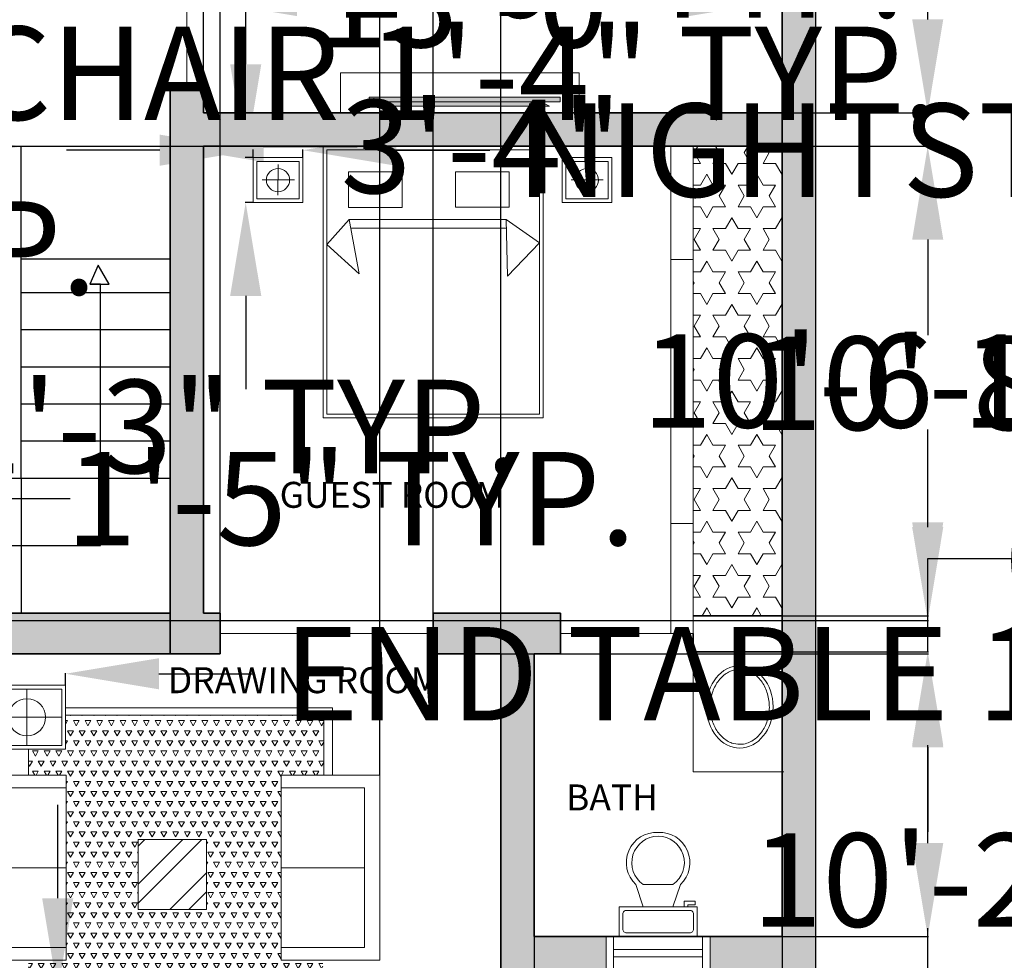
# Model space of a CAD drawing. Units: inches. Extents: x 29 to 6336, y 3 to 2592.
# Tile 6 of 8: x 5672 to 5938, y 2100 to 2354. Entities that reach past the tile are written whole.
import ezdxf

# ---------------------------------------------------------------- set-up
doc = ezdxf.new("R2010")
doc.units = ezdxf.units.IN
doc.header["$MEASUREMENT"] = 0
for name, color, linetype, lineweight in [('A-ANNO-DIMS', 2, 'Continuous', 18), ('A-AREA-IDEN', 7, 'Continuous', 18), ('A-DOOR', 4, 'Continuous', 18), ('A-FLOR-CASE', 8, 'Continuous', 18), ('A-FLOR-FIXT', 8, 'Continuous', 18), ('A-FLOR-FIXT-PATT', 9, 'Continuous', 13), ('A-FLOR-PATT', 9, 'Continuous', 13), ('A-FLOR-STRS', 7, 'Continuous', 25), ('A-FURN', 8, 'Continuous', 18), ('A-FURN-PATT', 18, 'Continuous', 13), ('A-GLAZ', 116, 'Continuous', 18), ('A-WALL', 7, 'Continuous', 35), ('A-WALL-PATT', 242, 'Continuous', 13), ('C-PROP', 7, 'Continuous', 25)]:
    doc.layers.add(name, color=color, linetype=linetype, lineweight=lineweight)
doc.styles.get("Standard").update_dxf_attribs({"font": 'arial.ttf'})
doc.dimstyles.get("Standard").update_dxf_attribs({"dimtxt": 25.18, "dimasz": 25.18, "dimexe": 0.18, "dimexo": 0.0625, "dimgap": 0.09, "dimtad": 0, "dimtih": 1, "dimtoh": 1, "dimdec": 0, "dimzin": 0, "dimdsep": 46, "dimlunit": 3, "dimtxsty": 'Standard', "dimcen": 0.09, "dimadec": 0, "dimazin": 0, "dimtfac": 1, "dimtdec": 0, "dimtofl": 0, "dimtmove": 0, "dimatfit": 3, "dimfxl": 1, "dimtolj": 1, "dimtzin": 0, "dimarcsym": 0})

# ---------------------------------------------------------------- blocks, each defined once
blk = doc.blocks.new('*U4')
for p, q in [((9.5, -6), (9.5, -2)), ((-10, -8.5), (-8, -8.5)), ((-10, -9.5), (-10, -8.5)), ((-7, -9.5), (-10, -9.5)), ((-8, -8.5), (-8, -8)), ((-7, -8), (-7, -9.5)), ((-4, -8), (-6, -14)), ((4, -8), (6, -14)), ((4, -14), (-4, -14))]:
    blk.add_line(p, q)
blk.add_lwpolyline([(10.5, -8), (10.5, 0), (-10.5, 0), (-10.5, -8)], close=True)
for points in [[(-9.5, -2), (-9.5, -6)], [(8.5, -1), (-8.5, -1)], [(-8.5, -7), (8.5, -7)]]:
    blk.add_lwpolyline(points)
for centre, radius, start, end in [((-8.625, -1.875), 0.8839, 81.8699, 188.1301), ((8.625, -1.875), 0.8839, 351.8699, 98.1301), ((-8.625, -6.125), 0.8839, 171.869898, 278.1301), ((8.625, -6.125), 0.8839, 261.8699, 8.1301), ((-0.4772, -19.9188), 8.0953, 133.01722, 273.38), ((0.0374, -19.8731), 7.127, 124.50543, 269.7), ((-0.0373, -19.8731), 7.127, 270.3, 55.4946), ((0.4773, -19.9188), 8.0953, 266.62, 46.9828)]:
    blk.add_arc(centre, radius, start, end)
blk = doc.blocks.new('WIN-24')
for p, q in [((0, 9), (0, 0)), ((2, 9), (2, 0)), ((26, 9), (26, 0)), ((28, 9), (28, 0)), ((2, 5.5), (26, 5.5)), ((2, 3.5), (26, 3.5))]:
    blk.add_line(p, q)
blk = doc.blocks.new('SOFA-TWO-SEAT')
blk.add_line((4.12, 24.97), (26.62, 24.97))
for points in [[(4.17, 49.94), (0, 49.94), (0, 0), (4.17, 0)], [(4.17, 49.94), (26.62, 49.94), (26.62, 46.51), (4.17, 46.51)], [(4.17, 3.43), (4.17, 46.51)], [(4.12, 3.43), (26.57, 3.43), (26.57, 0), (4.12, 0)]]:
    blk.add_lwpolyline(points)
blk.add_lwpolyline([(26.62, 46.51), (4.12, 46.51), (4.12, 3.43), (26.62, 3.43)], close=True)
blk = doc.blocks.new('NIGHTSTAND-13X12')
for p, q in [((6.7, 10.24), (6.69, 1.97)), ((2.43, 6.11), (11.1, 6.11))]:
    blk.add_line(p, q)
for points in [[(0, 12.1), (13.41, 12.1), (13.41, 0), (0, 0)], [(1, 11.1), (12.41, 11.1), (12.41, 1), (1, 1)]]:
    blk.add_lwpolyline(points, close=True)
blk.add_circle((6.7, 6.05), 3.13)
blk = doc.blocks.new('END-TABLE-21X17')
for p, q in [((10.41, 16.21), (10.41, 1)), ((1, 8.6), (19.81, 8.6))]:
    blk.add_line(p, q)
for points in [[(0, 17.21), (20.81, 17.21), (20.81, 0), (0, 0)], [(1, 16.21), (19.81, 16.21), (19.81, 1), (1, 1)]]:
    blk.add_lwpolyline(points, close=True)
blk.add_circle((10.41, 8.6), 5)
blk = doc.blocks.new('BASIN-VANITY')
for p, q in [((32.36, 0), (32.36, 24.47)), ((0, 0), (32.36, 0))]:
    blk.add_line(p, q)
blk.add_circle((14.85, 12.56), 0.667)
blk.add_ellipse((14.85, 12.56), major_axis=(11.1, 0), ratio=0.808824)
blk.add_open_spline([(24.95, 12.56), (24.95, 13.21), (24.85, 13.86), (24.35, 15.41), (23.86, 16.28), (22.49, 17.85), (21.62, 18.55), (19.61, 19.66), (18.47, 20.07), (16.07, 20.54), (14.82, 20.6), (12.37, 20.35), (11.18, 20.05), (9.01, 19.14), (8.04, 18.52), (6.44, 17.08), (5.81, 16.25), (4.97, 14.49), (4.75, 13.56), (4.73, 11.7), (4.93, 10.77), (5.73, 9), (6.33, 8.16), (7.89, 6.69), (8.85, 6.07), (10.99, 5.12), (12.18, 4.8), (14.62, 4.52), (15.88, 4.56), (18.29, 4.99), (19.44, 5.38), (21.47, 6.46), (22.36, 7.14), (23.77, 8.7), (24.29, 9.57), (24.83, 11.15), (24.95, 11.85), (24.95, 12.56)], degree=3, knots=[0, 0, 0, 0, 0.253102, 0.253102, 0.612978, 0.612978, 0.972853, 0.972853, 1.332728, 1.332728, 1.692603, 1.692603, 2.052478, 2.052478, 2.412354, 2.412354, 2.772229, 2.772229, 3.132104, 3.132104, 3.491979, 3.491979, 3.851854, 3.851854, 4.21173, 4.21173, 4.571605, 4.571605, 4.93148, 4.93148, 5.291355, 5.291355, 5.651231, 5.651231, 6.011106, 6.011106, 6.283185, 6.283185, 6.283185, 6.283185])
blk = doc.blocks.new('*D20')
at = {"layer": 'A-ANNO-DIMS', "color": 0, "lineweight": -2, "transparency": 16777216}
for p, q in [((5561.46, 2339.22), (5536.28, 2339.22)), ((5586.64, 2341.55), (5586.64, 2339.04)), ((5602.54, 2341.55), (5602.54, 2339.04)), ((5627.72, 2339.22), (5652.9, 2339.22))]:
    blk.add_line(p, q, dxfattribs=at)
at = {"layer": 'A-ANNO-DIMS', "color": 0, "transparency": 16777216}
for points in [[(5561.46, 2343.42), (5561.46, 2335.03), (5586.64, 2339.22)], [(5627.72, 2343.42), (5627.72, 2335.03), (5602.54, 2339.22)]]:
    blk.add_solid(points, dxfattribs=at)
at = {"layer": 'Defpoints', "color": 0, "transparency": 16777216}
for p in [(5586.64, 2341.61), (5602.54, 2341.61), (5602.54, 2339.22)]:
    blk.add_point(p, dxfattribs=at)
at = {"layer": 'A-ANNO-DIMS', "color": 0, "transparency": 16777216, "insert": (5789.2, 2339.22), "char_height": 25.18, "attachment_point": 5}
blk.add_mtext('\\A1;CHAIR 1\'-4" TYP.', dxfattribs=at)
blk = doc.blocks.new('*D21')
at = {"layer": 'A-ANNO-DIMS', "color": 0, "lineweight": -2, "transparency": 16777216}
for p, q in [((5604.93, 2381.81), (5604.93, 2406.99)), ((5604.93, 2406.99), (5630.11, 2406.99)), ((5602.6, 2356.63), (5605.11, 2356.63)), ((5602.6, 2341.61), (5605.11, 2341.61)), ((5604.93, 2316.43), (5604.93, 2291.25))]:
    blk.add_line(p, q, dxfattribs=at)
at = {"layer": 'A-ANNO-DIMS', "color": 0, "transparency": 16777216}
for points in [[(5600.73, 2381.81), (5609.12, 2381.81), (5604.93, 2356.63)], [(5600.73, 2316.43), (5609.12, 2316.43), (5604.93, 2341.61)]]:
    blk.add_solid(points, dxfattribs=at)
at = {"layer": 'Defpoints', "color": 0, "transparency": 16777216}
for p in [(5602.54, 2356.63), (5604.93, 2356.63), (5602.54, 2341.61)]:
    blk.add_point(p, dxfattribs=at)
at = {"layer": 'A-ANNO-DIMS', "color": 0, "transparency": 16777216, "insert": (5705.75, 2406.99), "char_height": 25.18, "attachment_point": 5}
blk.add_mtext('\\A1;1\'-3" TYP.', dxfattribs=at)
blk = doc.blocks.new('*D24')
at = {"layer": 'A-ANNO-DIMS', "color": 0, "lineweight": -2, "transparency": 16777216}
for p, q in [((5412.73, 2243.97), (5387.55, 2243.97)), ((5437.91, 2241.81), (5437.91, 2244.15)), ((5452.73, 2241.81), (5452.73, 2244.15)), ((5477.91, 2243.97), (5503.09, 2243.97))]:
    blk.add_line(p, q, dxfattribs=at)
at = {"layer": 'A-ANNO-DIMS', "color": 0, "transparency": 16777216}
for points in [[(5412.73, 2248.16), (5412.73, 2239.77), (5437.91, 2243.97)], [(5477.91, 2248.16), (5477.91, 2239.77), (5452.73, 2243.97)]]:
    blk.add_solid(points, dxfattribs=at)
at = {"layer": 'Defpoints', "color": 0, "transparency": 16777216}
for p in [(5452.73, 2243.97), (5437.91, 2241.74), (5452.73, 2241.74)]:
    blk.add_point(p, dxfattribs=at)
at = {"layer": 'A-ANNO-DIMS', "color": 0, "transparency": 16777216, "insert": (5658.52, 2243.97), "char_height": 25.18, "attachment_point": 5}
blk.add_mtext('\\A1;BURNER 1\'-3" TYP.', dxfattribs=at)
blk = doc.blocks.new('*D25')
at = {"layer": 'A-ANNO-DIMS', "color": 0, "lineweight": -2, "transparency": 16777216}
for p, q in [((5435.68, 2266.92), (5435.68, 2292.1)), ((5435.68, 2292.1), (5460.86, 2292.1)), ((5437.84, 2241.74), (5435.5, 2241.74)), ((5437.84, 2231.12), (5435.5, 2231.12)), ((5435.68, 2205.94), (5435.68, 2180.76))]:
    blk.add_line(p, q, dxfattribs=at)
at = {"layer": 'A-ANNO-DIMS', "color": 0, "transparency": 16777216}
for points in [[(5431.49, 2266.92), (5439.88, 2266.92), (5435.68, 2241.74)], [(5431.49, 2205.94), (5439.88, 2205.94), (5435.68, 2231.12)]]:
    blk.add_solid(points, dxfattribs=at)
at = {"layer": 'Defpoints', "color": 0, "transparency": 16777216}
for p in [(5435.68, 2241.74), (5437.91, 2241.74), (5437.91, 2231.12)]:
    blk.add_point(p, dxfattribs=at)
at = {"layer": 'A-ANNO-DIMS', "color": 0, "transparency": 16777216, "insert": (5576.81, 2292.1), "char_height": 25.18, "attachment_point": 5}
blk.add_mtext('\\A1;0\'-10 1/2" TYP.', dxfattribs=at)
blk = doc.blocks.new('*D28')
at = {"layer": 'A-ANNO-DIMS', "color": 0, "lineweight": -2, "transparency": 16777216}
for p, q in [((5689.81, 2064.89), (5689.81, 2057.28)), ((5739.75, 2064.89), (5739.75, 2057.28)), ((5664.63, 2057.46), (5639.45, 2057.46)), ((5764.93, 2057.46), (5790.11, 2057.46))]:
    blk.add_line(p, q, dxfattribs=at)
at = {"layer": 'A-ANNO-DIMS', "color": 0, "transparency": 16777216}
for points in [[(5664.63, 2061.65), (5664.63, 2053.26), (5689.81, 2057.46)], [(5764.93, 2061.65), (5764.93, 2053.26), (5739.75, 2057.46)]]:
    blk.add_solid(points, dxfattribs=at)
at = {"layer": 'Defpoints', "color": 0, "transparency": 16777216}
for p in [(5689.81, 2064.95), (5739.75, 2064.95), (5689.81, 2057.46)]:
    blk.add_point(p, dxfattribs=at)
at = {"layer": 'A-ANNO-DIMS', "color": 0, "transparency": 16777216, "insert": (5509.91, 2057.46), "char_height": 25.18, "attachment_point": 5}
blk.add_mtext('\\A1;SOFA 4\'-2" TYP.', dxfattribs=at)
blk = doc.blocks.new('*D29')
at = {"layer": 'A-ANNO-DIMS', "color": 0, "lineweight": -2, "transparency": 16777216}
for p, q in [((5682.32, 2116.75), (5682.32, 2141.93)), ((5689.75, 2091.57), (5682.14, 2091.57)), ((5689.75, 2064.95), (5682.14, 2064.95)), ((5682.32, 2039.77), (5682.32, 2014.59))]:
    blk.add_line(p, q, dxfattribs=at)
at = {"layer": 'A-ANNO-DIMS', "color": 0, "transparency": 16777216}
for points in [[(5678.12, 2116.75), (5686.52, 2116.75), (5682.32, 2091.57)], [(5678.12, 2039.77), (5686.52, 2039.77), (5682.32, 2064.95)]]:
    blk.add_solid(points, dxfattribs=at)
at = {"layer": 'Defpoints', "color": 0, "transparency": 16777216}
for p in [(5682.32, 2091.57), (5689.81, 2091.57), (5689.81, 2064.95)]:
    blk.add_point(p, dxfattribs=at)
at = {"layer": 'A-ANNO-DIMS', "color": 0, "transparency": 16777216, "insert": (5682.32, 2078.26), "char_height": 25.18, "attachment_point": 5}
blk.add_mtext('\\A1;2\'-2 1/2" TYP.', dxfattribs=at)
blk = doc.blocks.new('*D32')
at = {"layer": 'A-ANNO-DIMS', "color": 0, "lineweight": -2, "transparency": 16777216}
for p, q in [((5709.84, 2318.47), (5684.66, 2318.47)), ((5735.02, 2316.52), (5735.02, 2318.65)), ((5748.43, 2316.52), (5748.43, 2318.65)), ((5773.61, 2318.47), (5798.79, 2318.47))]:
    blk.add_line(p, q, dxfattribs=at)
at = {"layer": 'A-ANNO-DIMS', "color": 0, "transparency": 16777216}
for points in [[(5709.84, 2322.67), (5709.84, 2314.27), (5735.02, 2318.47)], [(5773.61, 2322.67), (5773.61, 2314.27), (5748.43, 2318.47)]]:
    blk.add_solid(points, dxfattribs=at)
at = {"layer": 'Defpoints', "color": 0, "transparency": 16777216}
for p in [(5748.43, 2318.47), (5735.02, 2316.46), (5748.43, 2316.46)]:
    blk.add_point(p, dxfattribs=at)
at = {"layer": 'A-ANNO-DIMS', "color": 0, "transparency": 16777216, "insert": (6023.56, 2318.47), "char_height": 25.18, "attachment_point": 5}
blk.add_mtext('\\A1;NIGHTSTAND 1\'-1 1/2" TYP.', dxfattribs=at)
blk = doc.blocks.new('*D33')
at = {"layer": 'A-ANNO-DIMS', "color": 0, "lineweight": -2, "transparency": 16777216}
for p, q in [((5733.01, 2341.64), (5733.01, 2366.82)), ((5733.01, 2366.82), (5758.19, 2366.82)), ((5734.96, 2316.46), (5732.83, 2316.46)), ((5734.96, 2304.36), (5732.83, 2304.36)), ((5733.01, 2279.18), (5733.01, 2254))]:
    blk.add_line(p, q, dxfattribs=at)
at = {"layer": 'A-ANNO-DIMS', "color": 0, "transparency": 16777216}
for points in [[(5728.81, 2341.64), (5737.21, 2341.64), (5733.01, 2316.46)], [(5728.81, 2279.18), (5737.21, 2279.18), (5733.01, 2304.36)]]:
    blk.add_solid(points, dxfattribs=at)
at = {"layer": 'Defpoints', "color": 0, "transparency": 16777216}
for p in [(5733.01, 2316.46), (5735.02, 2316.46), (5735.02, 2304.36)]:
    blk.add_point(p, dxfattribs=at)
at = {"layer": 'A-ANNO-DIMS', "color": 0, "transparency": 16777216, "insert": (5833.84, 2366.82), "char_height": 25.18, "attachment_point": 5}
blk.add_mtext('\\A1;1\'-0" TYP.', dxfattribs=at)
blk = doc.blocks.new('*D34')
at = {"layer": 'A-ANNO-DIMS', "color": 0, "lineweight": -2, "transparency": 16777216}
for p, q in [((5638.44, 2177.3), (5613.26, 2177.3)), ((5663.62, 2174.24), (5663.62, 2177.48)), ((5684.43, 2174.24), (5684.43, 2177.48)), ((5709.61, 2177.3), (5734.79, 2177.3))]:
    blk.add_line(p, q, dxfattribs=at)
at = {"layer": 'A-ANNO-DIMS', "color": 0, "transparency": 16777216}
for points in [[(5638.44, 2181.49), (5638.44, 2173.1), (5663.62, 2177.3)], [(5709.61, 2181.49), (5709.61, 2173.1), (5684.43, 2177.3)]]:
    blk.add_solid(points, dxfattribs=at)
at = {"layer": 'Defpoints', "color": 0, "transparency": 16777216}
for p in [(5684.43, 2177.3), (5663.62, 2174.18), (5684.43, 2174.18)]:
    blk.add_point(p, dxfattribs=at)
at = {"layer": 'A-ANNO-DIMS', "color": 0, "transparency": 16777216, "insert": (5913.59, 2177.3), "char_height": 25.18, "attachment_point": 5}
blk.add_mtext('\\A1;END TABLE 1\'-9" TYP.', dxfattribs=at)
blk = doc.blocks.new('*D35')
at = {"layer": 'A-ANNO-DIMS', "color": 0, "lineweight": -2, "transparency": 16777216}
for p, q in [((5660.5, 2199.36), (5660.5, 2224.54)), ((5660.5, 2224.54), (5685.68, 2224.54)), ((5663.56, 2174.18), (5660.32, 2174.18)), ((5663.56, 2156.97), (5660.32, 2156.97)), ((5660.5, 2131.79), (5660.5, 2106.61))]:
    blk.add_line(p, q, dxfattribs=at)
at = {"layer": 'A-ANNO-DIMS', "color": 0, "transparency": 16777216}
for points in [[(5656.3, 2199.36), (5664.7, 2199.36), (5660.5, 2174.18)], [(5656.3, 2131.79), (5664.7, 2131.79), (5660.5, 2156.97)]]:
    blk.add_solid(points, dxfattribs=at)
at = {"layer": 'Defpoints', "color": 0, "transparency": 16777216}
for p in [(5660.5, 2174.18), (5663.62, 2174.18), (5663.62, 2156.97)]:
    blk.add_point(p, dxfattribs=at)
at = {"layer": 'A-ANNO-DIMS', "color": 0, "transparency": 16777216, "insert": (5761.33, 2224.54), "char_height": 25.18, "attachment_point": 5}
blk.add_mtext('\\A1;1\'-5" TYP.', dxfattribs=at)
blk = doc.blocks.new('*D45')
at = {"layer": 'A-ANNO-DIMS', "color": 0, "lineweight": -2, "transparency": 16777216}
for p, q in [((5721.66, 2328.63), (5721.66, 2358.99)), ((5746.84, 2358.81), (5757.5, 2358.81)), ((5852.48, 2358.81), (5841.81, 2358.81)), ((5877.66, 2328.63), (5877.66, 2358.99))]:
    blk.add_line(p, q, dxfattribs=at)
at = {"layer": 'A-ANNO-DIMS', "color": 0, "transparency": 16777216}
for points in [[(5746.84, 2363.01), (5746.84, 2354.62), (5721.66, 2358.81)], [(5852.48, 2363.01), (5852.48, 2354.62), (5877.66, 2358.81)]]:
    blk.add_solid(points, dxfattribs=at)
at = {"layer": 'Defpoints', "color": 0, "transparency": 16777216}
for p in [(5877.66, 2358.81), (5721.66, 2328.56), (5877.66, 2328.56)]:
    blk.add_point(p, dxfattribs=at)
at = {"layer": 'A-ANNO-DIMS', "color": 0, "transparency": 16777216, "insert": (5799.66, 2358.81), "char_height": 25.18, "attachment_point": 5}
blk.add_mtext('\\A1;13\'-0"', dxfattribs=at)
blk = doc.blocks.new('*D46')
at = {"layer": 'A-ANNO-DIMS', "color": 0, "lineweight": -2, "transparency": 16777216}
for p, q in [((5877.72, 2483.33), (5917.09, 2483.33)), ((5916.91, 2458.15), (5916.91, 2418.68)), ((5916.91, 2353.74), (5916.91, 2393.21)), ((5877.72, 2328.56), (5917.09, 2328.56))]:
    blk.add_line(p, q, dxfattribs=at)
at = {"layer": 'A-ANNO-DIMS', "color": 0, "transparency": 16777216}
for points in [[(5912.71, 2458.15), (5921.1, 2458.15), (5916.91, 2483.33)], [(5912.71, 2353.74), (5921.1, 2353.74), (5916.91, 2328.56)]]:
    blk.add_solid(points, dxfattribs=at)
at = {"layer": 'Defpoints', "color": 0, "transparency": 16777216}
for p in [(5877.66, 2483.33), (5916.91, 2483.33), (5877.66, 2328.56)]:
    blk.add_point(p, dxfattribs=at)
at = {"layer": 'A-ANNO-DIMS', "color": 0, "transparency": 16777216, "insert": (5916.91, 2405.95), "char_height": 25.18, "attachment_point": 5}
blk.add_mtext('\\A1;12\'-11"', dxfattribs=at)
blk = doc.blocks.new('*D50')
at = {"layer": 'A-ANNO-DIMS', "color": 0, "lineweight": -2, "transparency": 16777216}
for p, q in [((5510.17, 2319.56), (5917.09, 2319.56)), ((5916.91, 2294.38), (5916.91, 2268.55)), ((5916.91, 2216.83), (5916.91, 2242.66)), ((5510.17, 2191.65), (5917.09, 2191.65))]:
    blk.add_line(p, q, dxfattribs=at)
at = {"layer": 'A-ANNO-DIMS', "color": 0, "transparency": 16777216}
for points in [[(5912.71, 2294.38), (5921.1, 2294.38), (5916.91, 2319.56)], [(5912.71, 2216.83), (5921.1, 2216.83), (5916.91, 2191.65)]]:
    blk.add_solid(points, dxfattribs=at)
at = {"layer": 'Defpoints', "color": 0, "transparency": 16777216}
for p in [(5510.11, 2319.56), (5916.91, 2319.56), (5510.11, 2191.65)]:
    blk.add_point(p, dxfattribs=at)
at = {"layer": 'A-ANNO-DIMS', "color": 0, "transparency": 16777216, "insert": (5916.91, 2255.61), "char_height": 25.18, "attachment_point": 5}
blk.add_mtext('\\A1;10\'-8"', dxfattribs=at)
blk = doc.blocks.new('*D51')
at = {"layer": 'A-ANNO-DIMS', "color": 0, "lineweight": -2, "transparency": 16777216}
for p, q in [((5877.72, 2319.56), (5917.09, 2319.56)), ((5916.91, 2294.38), (5916.91, 2269.37)), ((5916.91, 2218.13), (5916.91, 2243.15)), ((5877.72, 2192.95), (5917.09, 2192.95))]:
    blk.add_line(p, q, dxfattribs=at)
at = {"layer": 'A-ANNO-DIMS', "color": 0, "transparency": 16777216}
for points in [[(5912.71, 2294.38), (5921.1, 2294.38), (5916.91, 2319.56)], [(5912.71, 2218.13), (5921.1, 2218.13), (5916.91, 2192.95)]]:
    blk.add_solid(points, dxfattribs=at)
at = {"layer": 'Defpoints', "color": 0, "transparency": 16777216}
for p in [(5877.66, 2319.56), (5916.91, 2319.56), (5877.66, 2192.95)]:
    blk.add_point(p, dxfattribs=at)
at = {"layer": 'A-ANNO-DIMS', "color": 0, "transparency": 16777216, "insert": (5916.91, 2256.26), "char_height": 25.18, "attachment_point": 5}
blk.add_mtext('\\A1;10\'-6 1/2"', dxfattribs=at)
blk = doc.blocks.new('*D53')
at = {"layer": 'A-ANNO-DIMS', "color": 0, "lineweight": -2, "transparency": 16777216}
for p, q in [((5801.82, 2182.65), (5917.09, 2182.65)), ((5916.91, 2157.47), (5916.91, 2134.63)), ((5916.91, 2085.9), (5916.91, 2108.74)), ((5801.82, 2060.72), (5917.09, 2060.72))]:
    blk.add_line(p, q, dxfattribs=at)
at = {"layer": 'A-ANNO-DIMS', "color": 0, "transparency": 16777216}
for points in [[(5912.71, 2157.47), (5921.1, 2157.47), (5916.91, 2182.65)], [(5912.71, 2085.9), (5921.1, 2085.9), (5916.91, 2060.72)]]:
    blk.add_solid(points, dxfattribs=at)
at = {"layer": 'Defpoints', "color": 0, "transparency": 16777216}
for p in [(5801.76, 2182.65), (5916.91, 2182.65), (5801.76, 2060.72)]:
    blk.add_point(p, dxfattribs=at)
at = {"layer": 'A-ANNO-DIMS', "color": 0, "transparency": 16777216, "insert": (5916.91, 2121.68), "char_height": 25.18, "attachment_point": 5}
blk.add_mtext('\\A1;10\'-2"', dxfattribs=at)
blk = doc.blocks.new('*D54')
at = {"layer": 'A-ANNO-DIMS', "color": 0, "lineweight": -2, "transparency": 16777216}
for p, q in [((5916.91, 2183.22), (5916.91, 2208.4)), ((5916.91, 2208.4), (5942.09, 2208.4)), ((5877.72, 2183.22), (5917.09, 2183.22)), ((5916.91, 2131.66), (5916.91, 2158.04)), ((5877.72, 2106.48), (5917.09, 2106.48))]:
    blk.add_line(p, q, dxfattribs=at)
at = {"layer": 'A-ANNO-DIMS', "color": 0, "transparency": 16777216}
for points in [[(5912.71, 2158.04), (5921.1, 2158.04), (5916.91, 2183.22)], [(5912.71, 2131.66), (5921.1, 2131.66), (5916.91, 2106.48)]]:
    blk.add_solid(points, dxfattribs=at)
at = {"layer": 'Defpoints', "color": 0, "transparency": 16777216}
for p in [(5877.66, 2183.22), (5916.91, 2183.22), (5877.66, 2106.48)]:
    blk.add_point(p, dxfattribs=at)
at = {"layer": 'A-ANNO-DIMS', "color": 0, "transparency": 16777216, "insert": (6005.05, 2208.4), "char_height": 25.18, "attachment_point": 5}
blk.add_mtext('\\A1;6\'-4 1/2"', dxfattribs=at)
blk = doc.blocks.new('*D55')
at = {"layer": 'A-ANNO-DIMS', "color": 0, "lineweight": -2, "transparency": 16777216}
for p, q in [((5810.76, 2106.42), (5810.76, 1921.9)), ((5877.66, 2106.42), (5877.66, 1921.9)), ((5835.94, 1922.08), (5852.48, 1922.08)), ((5877.66, 1922.08), (5902.84, 1922.08))]:
    blk.add_line(p, q, dxfattribs=at)
at = {"layer": 'A-ANNO-DIMS', "color": 0, "transparency": 16777216}
for points in [[(5835.94, 1926.28), (5835.94, 1917.88), (5810.76, 1922.08)], [(5852.48, 1926.28), (5852.48, 1917.88), (5877.66, 1922.08)]]:
    blk.add_solid(points, dxfattribs=at)
at = {"layer": 'Defpoints', "color": 0, "transparency": 16777216}
for p in [(5810.76, 2106.48), (5877.66, 2106.48), (5877.66, 1922.08)]:
    blk.add_point(p, dxfattribs=at)
at = {"layer": 'A-ANNO-DIMS', "color": 0, "transparency": 16777216, "insert": (5936.39, 1922.08), "char_height": 25.18, "attachment_point": 5}
blk.add_mtext('\\A1;5\'-7"', dxfattribs=at)
blk = doc.blocks.new('*D60')
at = {"layer": 'A-ANNO-DIMS', "color": 0, "lineweight": -2, "transparency": 16777216}
for p, q in [((5647.28, 2319.47), (5622.1, 2319.47)), ((5672.46, 2289.28), (5672.46, 2319.65)), ((5712.66, 2289.28), (5712.66, 2319.65)), ((5737.84, 2319.47), (5763.02, 2319.47))]:
    blk.add_line(p, q, dxfattribs=at)
at = {"layer": 'A-ANNO-DIMS', "color": 0, "transparency": 16777216}
for points in [[(5647.28, 2323.67), (5647.28, 2315.27), (5672.46, 2319.47)], [(5737.84, 2323.67), (5737.84, 2315.27), (5712.66, 2319.47)]]:
    blk.add_solid(points, dxfattribs=at)
at = {"layer": 'Defpoints', "color": 0, "transparency": 16777216}
for p in [(5712.66, 2319.47), (5672.46, 2289.22), (5712.66, 2289.22)]:
    blk.add_point(p, dxfattribs=at)
at = {"layer": 'A-ANNO-DIMS', "color": 0, "transparency": 16777216, "insert": (5796.57, 2319.47), "char_height": 25.18, "attachment_point": 5}
blk.add_mtext('\\A1;3\'-4"', dxfattribs=at)
blk = doc.blocks.new('*D65')
at = {"layer": 'A-ANNO-DIMS', "color": 0, "lineweight": -2, "transparency": 16777216}
for p, q in [((5726.12, 2182.71), (5726.12, 2522.76)), ((5751.3, 2522.58), (5758.41, 2522.58)), ((5783.59, 2182.71), (5783.59, 2522.76)), ((5783.59, 2522.58), (5808.77, 2522.58))]:
    blk.add_line(p, q, dxfattribs=at)
at = {"layer": 'A-ANNO-DIMS', "color": 0, "transparency": 16777216}
for points in [[(5751.3, 2526.78), (5751.3, 2518.38), (5726.12, 2522.58)], [(5758.41, 2526.78), (5758.41, 2518.38), (5783.59, 2522.58)]]:
    blk.add_solid(points, dxfattribs=at)
at = {"layer": 'Defpoints', "color": 0, "transparency": 16777216}
for p in [(5783.59, 2522.58), (5726.12, 2182.65), (5783.59, 2182.65)]:
    blk.add_point(p, dxfattribs=at)
at = {"layer": 'A-ANNO-DIMS', "color": 0, "transparency": 16777216, "insert": (5872.17, 2522.58), "char_height": 25.18, "attachment_point": 5}
blk.add_mtext('\\A1;4\'-9 1/2"', dxfattribs=at)
blk = doc.blocks.new('*D67')
at = {"layer": 'A-ANNO-DIMS', "color": 0, "lineweight": -2, "transparency": 16777216}
for p, q in [((5743.99, 2522.58), (5718.81, 2522.58)), ((5769.17, 2150.03), (5769.17, 2522.76)), ((5801.76, 2182.71), (5801.76, 2522.76)), ((5826.94, 2522.58), (5852.12, 2522.58))]:
    blk.add_line(p, q, dxfattribs=at)
at = {"layer": 'A-ANNO-DIMS', "color": 0, "transparency": 16777216}
for points in [[(5743.99, 2526.78), (5743.99, 2518.38), (5769.17, 2522.58)], [(5826.94, 2526.78), (5826.94, 2518.38), (5801.76, 2522.58)]]:
    blk.add_solid(points, dxfattribs=at)
at = {"layer": 'Defpoints', "color": 0, "transparency": 16777216}
for p in [(5801.76, 2522.58), (5801.76, 2182.65), (5769.17, 2149.97)]:
    blk.add_point(p, dxfattribs=at)
at = {"layer": 'A-ANNO-DIMS', "color": 0, "transparency": 16777216, "insert": (5915.23, 2522.58), "char_height": 25.18, "attachment_point": 5}
blk.add_mtext('\\A1;2\'-8 1/2"', dxfattribs=at)
blk = doc.blocks.new('*D71')
at = {"layer": 'A-ANNO-DIMS', "color": 0, "lineweight": -2, "transparency": 16777216}
for p, q in [((5510.6, 2313.41), (5548.31, 2313.41)), ((5835.74, 2313.41), (5835.92, 2313.41)), ((5835.83, 2313.32), (5835.83, 2313.5))]:
    blk.add_line(p, q, dxfattribs=at)
at = {"layer": 'A-ANNO-DIMS', "color": 0, "transparency": 16777216}
blk.add_solid([(5548.31, 2317.61), (5548.31, 2309.22), (5573.49, 2313.41)], dxfattribs=at)
at = {"layer": 'Defpoints', "color": 0, "transparency": 16777216}
for p in [(5573.49, 2313.41), (5835.83, 2313.41)]:
    blk.add_point(p, dxfattribs=at)
at = {"layer": 'A-ANNO-DIMS', "color": 0, "transparency": 16777216, "insert": (5416.09, 2313.41), "char_height": 25.18, "attachment_point": 5}
blk.add_mtext('\\A1;R21\'-10 1/2"', dxfattribs=at)

msp = doc.modelspace()

# ---------------------------------------------------------------- hatches: boundary and pattern name
at = {"layer": 'A-FLOR-FIXT-PATT'}
h = msp.add_hatch(dxfattribs=at)
h.set_pattern_fill('STARS', color=256, scale=27)
h.paths.add_polyline_path([(5877.66, 2319.56), (5853.66, 2319.56), (5853.66, 2192.95), (5877.66, 2192.95)])
at = {"layer": 'A-FLOR-PATT'}
h = msp.add_hatch(dxfattribs=at)
h.set_pattern_fill('TRIANG', color=256, scale=8.4)
h.paths.add_polyline_path([(5742.55, 2146.54), (5742.55, 2149.97), (5754.06, 2149.97), (5754.06, 2166.16), (5684.43, 2166.16), (5684.43, 2156.97), (5674.45, 2156.97), (5674.45, 2149.97), (5684.63, 2149.97), (5684.63, 2146.54), (5684.63, 2103.46), (5684.58, 2103.46), (5684.58, 2100.03), (5674.45, 2100.03), (5674.45, 2091.34), (5682.83, 2091.34), (5682.83, 2084.5), (5689.81, 2084.5), (5689.81, 2091.57), (5693.24, 2091.57), (5736.32, 2091.57), (5736.32, 2091.52), (5739.75, 2091.52), (5739.75, 2079.85), (5753.82, 2079.85), (5753.82, 2100.03), (5742.6, 2100.03), (5742.6, 2103.46), (5742.55, 2103.46)])
h.paths.add_polyline_path([(5722.48, 2132.65), (5722.48, 2113.77), (5704, 2113.77), (5704, 2132.65)], flags=16)
at = {"layer": 'A-FURN-PATT'}
h = msp.add_hatch(color=256, dxfattribs=at)
h.dxf.hatch_style = 1
h.paths.add_polyline_path([(5817.77, 2332.76), (5766.3, 2332.76), (5766.3, 2331.51), (5817.77, 2331.51)])
h.paths.add_polyline_path([(5812.71, 2331.51), (5769.48, 2331.51), (5768.17, 2330.33), (5814.94, 2330.33)])
h = msp.add_hatch(dxfattribs=at)
h.set_pattern_fill('ANSI32', color=256, scale=29)
h.paths.add_polyline_path([(5722.48, 2132.65), (5704, 2132.65), (5704, 2113.77), (5722.48, 2113.77)])
at = {"layer": 'A-WALL-PATT'}
h = msp.add_hatch(color=256, dxfattribs=at)
h.dxf.hatch_style = 1
h.paths.add_polyline_path([(5558.68, 2492.33), (5459.71, 2492.33), (5459.71, 2483.33), (5511.77, 2483.33), (5511.77, 2388.68), (5520.77, 2388.68), (5520.77, 2393.05), (5526.31, 2393.05), (5526.31, 2402.05), (5520.77, 2402.05), (5520.77, 2483.33), (5558.68, 2483.33)])
h.paths.add_polyline_path([(5659.13, 2492.33), (5586.68, 2492.33), (5586.68, 2483.33), (5624.6, 2483.33), (5624.6, 2402.05), (5562.29, 2402.05), (5562.29, 2393.05), (5676.48, 2393.05), (5676.48, 2402.05), (5633.6, 2402.05), (5633.6, 2422.71), (5633.6, 2483.33), (5659.13, 2483.33)])
h.paths.add_polyline_path([(5886.66, 2492.33), (5687.13, 2492.33), (5687.13, 2483.33), (5712.66, 2483.33), (5712.66, 2468.69), (5721.66, 2468.69), (5721.66, 2483.33), (5877.66, 2483.33), (5877.66, 2106.48), (5858.21, 2106.48), (5858.21, 2097.48), (5877.66, 2097.48), (5877.66, 1961.33), (5877.66, 1952.33), (5886.66, 1952.33)])
h.paths.add_polyline_path([(5721.66, 2416.69), (5712.66, 2416.69), (5712.66, 2402.05), (5709.45, 2402.05), (5709.45, 2393.05), (5712.66, 2393.05), (5712.66, 2386.01), (5721.66, 2386.01)], flags=17)
h.paths.add_polyline_path([(5355.66, 2483.33), (5407.71, 2483.33), (5407.71, 2492.33), (5346.66, 2492.33), (5346.66, 2431.95), (5355.66, 2431.95)])
h.paths.add_polyline_path([(5355.66, 2379.95), (5346.66, 2379.95), (5346.66, 2319.56), (5355.66, 2319.56), (5355.66, 2328.56)])
h.paths.add_polyline_path([(5520.77, 2337.13), (5511.77, 2337.13), (5511.77, 2328.56), (5410.6, 2328.56), (5410.6, 2319.56), (5410.6, 2281.61), (5419.6, 2281.61), (5419.6, 2319.56), (5510.11, 2319.56), (5510.11, 2234.67), (5519.11, 2234.67), (5519.11, 2319.56), (5520.77, 2319.56)])
h.paths.add_polyline_path([(5519.11, 2197.33), (5510.11, 2197.33), (5510.11, 2191.65), (5419.6, 2191.65), (5419.6, 2228.6), (5419.6, 2229.61), (5410.6, 2229.61), (5410.6, 2182.65), (5519.11, 2182.65)])
h.paths.add_polyline_path([(5712.66, 2193.6), (5592.36, 2193.6), (5592.36, 2182.65), (5624.77, 2182.65), (5633.77, 2182.65), (5712.66, 2182.65)])
h.paths.add_polyline_path([(5633.77, 2182.65), (5624.77, 2182.65), (5624.77, 2051.72), (5633.77, 2051.72), (5691.77, 2051.72), (5691.77, 2060.72), (5633.77, 2060.72)])
h.paths.add_polyline_path([(5810.76, 2097.48), (5830.21, 2097.48), (5830.21, 2106.48), (5810.76, 2106.48), (5810.76, 2182.65), (5817.87, 2182.65), (5817.87, 2193.6), (5783.59, 2193.6), (5783.59, 2182.65), (5801.76, 2182.65), (5801.76, 2060.72), (5743.77, 2060.72), (5743.77, 2051.72), (5810.76, 2051.72)], flags=17)
h.paths.add_polyline_path([(5721.66, 2319.56), (5877.66, 2319.56), (5877.66, 2328.56), (5721.66, 2328.56), (5721.66, 2335.85), (5712.66, 2335.85), (5712.66, 2319.56), (5712.66, 2182.65), (5726.12, 2182.65), (5726.12, 2193.6), (5721.66, 2193.6)], flags=17)
h.paths.add_polyline_path([(5631.73, 2431.78), (5711.31, 2431.78), (5711.31, 2446.2), (5631.73, 2446.2)], flags=9)

# ---------------------------------------------------------------- linework, layer by layer
at = {"layer": 'A-DOOR'}
for p, q in [((5717.16, 2386.01), (5717.16, 2335.85)), ((5726.12, 2188.13), (5783.59, 2188.13)), ((5817.87, 2188.13), (5853.66, 2188.13))]:
    msp.add_line(p, q, dxfattribs=at)
at = {"layer": 'A-FLOR-CASE'}
for p, q in [((5847.66, 2319.56), (5847.66, 2188.13)), ((5853.66, 2319.56), (5853.66, 2188.13)), ((5847.66, 2288.96), (5853.66, 2288.96)), ((5847.66, 2217.8), (5853.66, 2217.8))]:
    msp.add_line(p, q, dxfattribs=at)
at = {"layer": 'A-FLOR-PATT'}
for p, q in [((5684.43, 2168.09), (5755.1, 2168.09)), ((5755.1, 2168.09), (5756.4, 2168.09)), ((5756.4, 2168.09), (5756.4, 2149.97)), ((5684.43, 2166.16), (5754.06, 2166.16)), ((5754.06, 2166.16), (5754.06, 2149.97)), ((5674.45, 2149.97), (5674.45, 2156.97))]:
    msp.add_line(p, q, dxfattribs=at)
at = {"layer": 'A-FLOR-STRS'}
for p, q in [((5672.46, 2230.08), (5672.46, 2289.22)), ((5672.46, 2289.22), (5712.66, 2289.22)), ((5693.18, 2287.5), (5690.96, 2282.38)), ((5696.15, 2282.38), (5693.18, 2287.5)), ((5693.88, 2282.38), (5690.96, 2282.38)), ((5690.96, 2282.38), (5696.15, 2282.38)), ((5693.88, 2211.84), (5693.88, 2282.38)), ((5672.46, 2280.08), (5712.66, 2280.08)), ((5672.46, 2270.08), (5712.66, 2270.08)), ((5672.46, 2260.08), (5712.66, 2260.08)), ((5672.46, 2250.08), (5712.66, 2250.08)), ((5672.46, 2240.08), (5712.66, 2240.08)), ((5608.08, 2230.08), (5672.46, 2230.08)), ((5672.46, 2230.08), (5672.46, 2193.6)), ((5672.46, 2230.08), (5712.66, 2230.08)), ((5608.08, 2211.84), (5693.88, 2211.84))]:
    msp.add_line(p, q, dxfattribs=at)
at = {"layer": 'A-FURN'}
for p, q in [((5769.48, 2331.51), (5768.17, 2330.33)), ((5814.94, 2330.33), (5812.71, 2331.51)), ((5768.17, 2330.33), (5814.94, 2330.33)), ((5760.9, 2299.78), (5754.86, 2293.04)), ((5760.9, 2299.78), (5803.26, 2299.78)), ((5763.59, 2285.11), (5760.9, 2299.78)), ((5803.26, 2299.78), (5812.21, 2293.48)), ((5803.6, 2284.48), (5803.26, 2299.78)), ((5761.32, 2297.47), (5803.31, 2297.45)), ((5754.86, 2293.04), (5763.59, 2285.11)), ((5812.21, 2293.48), (5803.6, 2284.48))]:
    msp.add_line(p, q, dxfattribs=at)
for points in [[(5758.55, 2328.56), (5822.96, 2328.56), (5822.96, 2339.35), (5758.55, 2339.35)], [(5766.3, 2332.76), (5817.77, 2332.76), (5817.77, 2331.51), (5766.3, 2331.51)], [(5753.86, 2319.56), (5813.21, 2319.56), (5813.21, 2246.3), (5753.86, 2246.3)], [(5754.86, 2318.56), (5812.21, 2318.56), (5812.21, 2247.3), (5754.86, 2247.3)], [(5760.74, 2312.59), (5775.19, 2312.59), (5775.19, 2303.02), (5760.74, 2303.02)], [(5789.57, 2312.66), (5804.01, 2312.66), (5804.01, 2303.09), (5789.57, 2303.09)], [(5704, 2132.65), (5722.48, 2132.65), (5722.48, 2113.77), (5704, 2113.77)]]:
    msp.add_lwpolyline(points, close=True, dxfattribs=at)
at = {"layer": 'A-WALL'}
for p, q in [((5877.66, 2483.33), (5877.66, 2106.48)), ((5721.66, 2335.85), (5712.66, 2335.85)), ((5712.66, 2335.85), (5712.66, 2182.65)), ((5712.66, 2335.85), (5712.66, 2319.56)), ((5721.66, 2335.85), (5721.66, 2328.56)), ((5721.66, 2335.85), (5721.66, 2328.56)), ((5721.66, 2328.56), (5877.66, 2328.56)), ((5721.66, 2319.56), (5877.66, 2319.56)), ((5721.66, 2319.56), (5721.66, 2193.6)), ((5592.36, 2193.6), (5712.66, 2193.6)), ((5721.66, 2193.6), (5726.12, 2193.6)), ((5726.12, 2193.6), (5726.12, 2182.65)), ((5783.59, 2193.6), (5783.59, 2182.65)), ((5783.59, 2193.6), (5817.87, 2193.6)), ((5817.87, 2182.65), (5817.87, 2193.6)), ((5877.66, 2192.95), (5853.66, 2192.95)), ((5853.66, 2188.13), (5853.66, 2183.22)), ((5633.77, 2182.65), (5712.66, 2182.65)), ((5712.66, 2182.65), (5726.12, 2182.65)), ((5783.59, 2182.65), (5801.76, 2182.65)), ((5801.76, 2182.65), (5801.76, 2060.72)), ((5810.76, 2182.65), (5810.76, 2106.48)), ((5810.76, 2182.65), (5817.87, 2182.65)), ((5877.66, 2183.22), (5853.66, 2183.22)), ((5810.76, 2106.48), (5877.66, 2106.48))]:
    msp.add_line(p, q, dxfattribs=at)
at = {"layer": 'C-PROP'}
msp.add_line((5886.66, 2492.33), (5886.66, 1952.33), dxfattribs=at)

# ---------------------------------------------------------------- block references
at = {"layer": 'A-FLOR-FIXT'}
for name, p, rotation in [('BASIN-VANITY', (5853.66, 2183.22), 270.0000000000001), ('*U4', (5844.21, 2106.48), 180)]:
    msp.add_blockref(name, p, dxfattribs=dict(at, rotation=rotation))
at = {"layer": 'A-FURN'}
for name, p in [('NIGHTSTAND-13X12', (5735.02, 2304.36)), ('NIGHTSTAND-13X12', (5818.3, 2304.36)), ('END-TABLE-21X17', (5663.62, 2156.97)), ('SOFA-TWO-SEAT', (5658, 2100.03))]:
    msp.add_blockref(name, p, dxfattribs=at)
at = {"layer": 'A-FURN', "extrusion": (0, 0, -1), "zscale": -1}
msp.add_blockref('SOFA-TWO-SEAT', (-5769.17, 2100.03), dxfattribs=at)
at = {"layer": 'A-GLAZ'}
msp.add_blockref('WIN-24', (5830.21, 2097.48), dxfattribs=at)

# ---------------------------------------------------------------- texts
at = {"layer": 'A-AREA-IDEN', "char_height": 7, "attachment_point": 1}
for s, width, heights, insert in [('GUEST ROOM', 80.6141, [0], (5742.16, 2229.04)), ('DRAWING ROOM', 94.6025, [7.24], (5712.02, 2179.06)), ('BATH', 54.3344, [0], (5819.39, 2147.45))]:
    msp.add_mtext_dynamic_manual_height_columns(s, width=width, gutter_width=1, heights=heights, dxfattribs=dict(at, insert=insert))

# ---------------------------------------------------------------- dimensions: what is measured, and where the dimension line sits
at = {"layer": 'A-ANNO-DIMS'}
for base, p1, p2, picture, middle in [((5801.76, 2522.58), (5769.17, 2149.97), (5801.76, 2182.65), '*D67', (5915.23, 2522.58)), ((5783.59, 2522.58), (5726.12, 2182.65), (5783.59, 2182.65), '*D65', (5872.17, 2522.58)), ((5877.66, 2358.81), (5721.66, 2328.56), (5877.66, 2328.56), '*D45', (5799.66, 2358.81)), ((5712.66, 2319.47), (5672.46, 2289.22), (5712.66, 2289.22), '*D60', (5796.57, 2319.47)), ((5877.66, 1922.08), (5810.76, 2106.48), (5877.66, 2106.48), '*D55', (5936.39, 1922.08))]:
    dim = msp.add_linear_dim(base=base, p1=p1, p2=p2, dimstyle='Standard', override={"dimdec": 1, "dimlfac": 1, "dimrnd": 0, "dimzin": 1, "dimdsep": 46, "dimlunit": 4, "dimfrac": 2}, dxfattribs=at)
    dim.commit()
    dim.dimension.update_dxf_attribs({"geometry": picture, "text_midpoint": middle})
for base, p1, p2, picture, middle in [((5916.91, 2483.33), (5877.66, 2328.56), (5877.66, 2483.33), '*D46', (5916.91, 2405.95)), ((5916.91, 2319.56), (5510.11, 2191.65), (5510.11, 2319.56), '*D50', (5916.91, 2255.61)), ((5916.91, 2319.56), (5877.66, 2192.95), (5877.66, 2319.56), '*D51', (5916.91, 2256.26)), ((5916.91, 2183.22), (5877.66, 2106.48), (5877.66, 2183.22), '*D54', (6005.05, 2208.4)), ((5916.91, 2182.65), (5801.76, 2060.72), (5801.76, 2182.65), '*D53', (5916.91, 2121.68))]:
    dim = msp.add_linear_dim(base=base, p1=p1, p2=p2, angle=90, dimstyle='Standard', override={"dimdec": 1, "dimlfac": 1, "dimrnd": 0, "dimzin": 1, "dimdsep": 46, "dimlunit": 4, "dimfrac": 2}, dxfattribs=at)
    dim.commit()
    dim.dimension.update_dxf_attribs({"geometry": picture, "text_midpoint": middle})
for base, p1, p2, angle, text, picture, middle in [((5604.93, 2356.63), (5602.54, 2341.61), (5602.54, 2356.63), 90, '<> TYP.', '*D21', (5705.75, 2406.99)), ((5733.01, 2316.46), (5735.02, 2304.36), (5735.02, 2316.46), 90, '<> TYP.', '*D33', (5833.84, 2366.82)), ((5435.68, 2241.74), (5437.91, 2231.12), (5437.91, 2241.74), 90, '<> TYP.', '*D25', (5576.81, 2292.1)), ((5660.5, 2174.18), (5663.62, 2156.97), (5663.62, 2174.18), 90, '<> TYP.', '*D35', (5761.33, 2224.54)), ((5682.32, 2091.57), (5689.81, 2064.95), (5689.81, 2091.57), 90, '<> TYP.', '*D29', (5682.32, 2078.26)), ((5689.81, 2057.46), (5739.75, 2064.95), (5689.81, 2064.95), 180, 'SOFA <> TYP.', '*D28', (5509.91, 2057.46))]:
    dim = msp.add_linear_dim(base=base, p1=p1, p2=p2, angle=angle, text=text, dimstyle='Standard', override={"dimdec": 1, "dimlfac": 1, "dimrnd": 0, "dimzin": 1, "dimdsep": 46, "dimlunit": 4, "dimfrac": 2}, dxfattribs=at)
    dim.commit()
    dim.dimension.update_dxf_attribs({"geometry": picture, "text_midpoint": middle})
for base, p1, p2, text, picture, middle in [((5602.54, 2339.22), (5586.64, 2341.61), (5602.54, 2341.61), 'CHAIR <> TYP.', '*D20', (5789.2, 2339.22)), ((5748.43, 2318.47), (5735.02, 2316.46), (5748.43, 2316.46), 'NIGHTSTAND <> TYP.', '*D32', (6023.56, 2318.47)), ((5452.73, 2243.97), (5437.91, 2241.74), (5452.73, 2241.74), 'BURNER <> TYP.', '*D24', (5658.52, 2243.97)), ((5684.43, 2177.3), (5663.62, 2174.18), (5684.43, 2174.18), 'END TABLE <> TYP.', '*D34', (5913.59, 2177.3))]:
    dim = msp.add_linear_dim(base=base, p1=p1, p2=p2, text=text, dimstyle='Standard', override={"dimdec": 1, "dimlfac": 1, "dimrnd": 0, "dimzin": 1, "dimdsep": 46, "dimlunit": 4, "dimfrac": 2}, dxfattribs=at)
    dim.commit()
    dim.dimension.update_dxf_attribs({"geometry": picture, "text_midpoint": middle})
dim = msp.add_radius_dim(center=(5835.83, 2313.41), mpoint=(5573.49, 2313.41), dimstyle='Standard', override={"dimdec": 1, "dimlfac": 1, "dimrnd": 0, "dimzin": 1, "dimdsep": 46, "dimlunit": 4, "dimfrac": 2}, dxfattribs=at)
dim.commit()
dim.dimension.update_dxf_attribs({"geometry": '*D71', "text_midpoint": (5416.09, 2313.41), "dimtype": 164})

doc.saveas('drawing.dxf')
